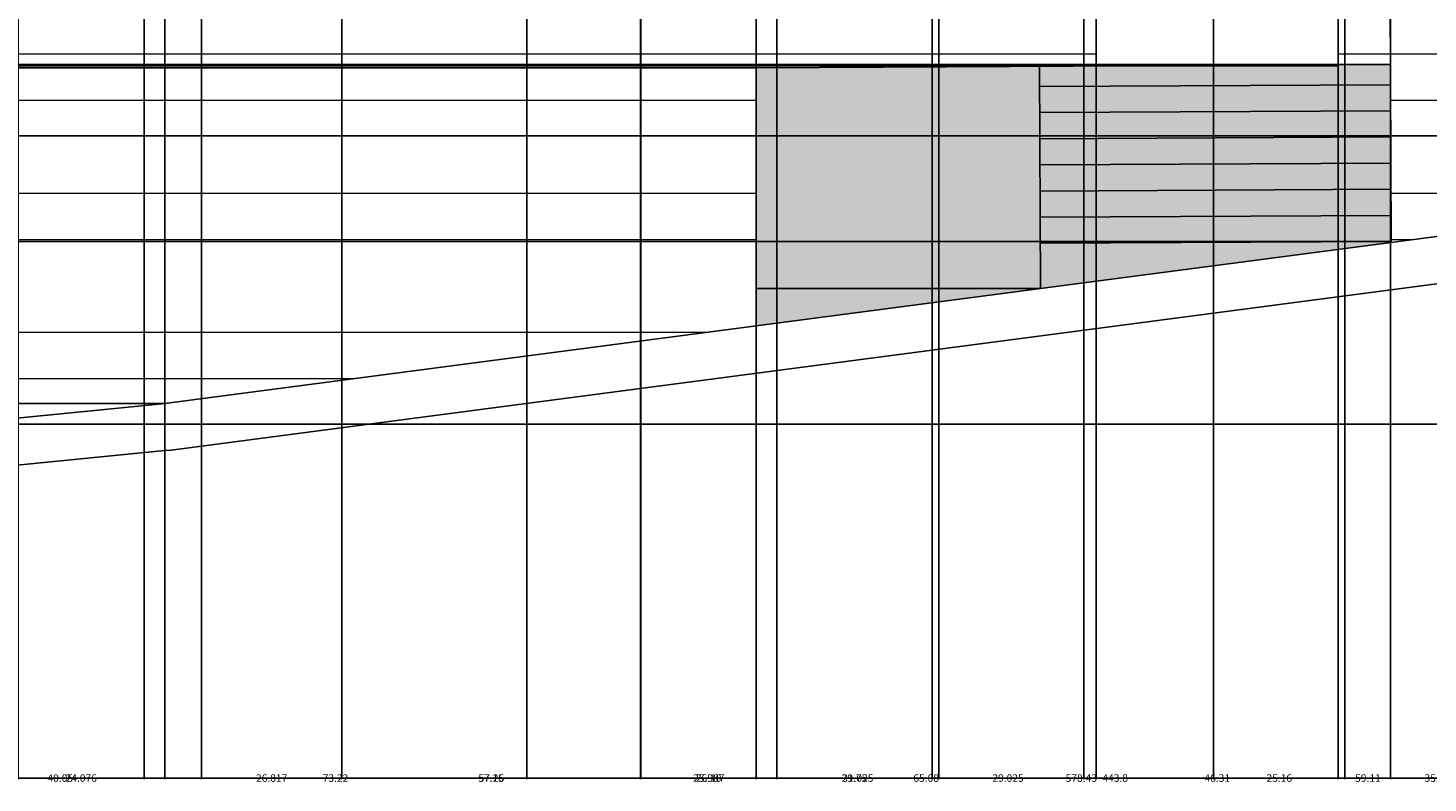
# Model space of a CAD drawing. Units: inches. Extents: x 241 to 943, y 109 to 1396.
# Tile 2 of 34: x 391 to 659, y 109 to 253. Entities that reach past the tile are written whole.
import ezdxf

# ---------------------------------------------------------------- set-up
doc = ezdxf.new("R2010")
doc.units = ezdxf.units.IN
doc.header["$MEASUREMENT"] = 0
for name, color, linetype, lineweight in [('A-ANNO-DIMS', 2, 'Continuous', 18), ('A-ELEV', 7, 'Continuous', 25), ('A-ELEV-SHAD', 9, 'Continuous', 13), ('A-GLAZ', 4, 'Continuous', 18), ('A-WALL-PATT', 8, 'Continuous', 13)]:
    doc.layers.add(name, color=color, linetype=linetype, lineweight=lineweight)
doc.styles.get("Standard").update_dxf_attribs({"font": 'arial.ttf'})
doc.dimstyles.get("Standard").update_dxf_attribs({"dimtxt": 1.4375, "dimasz": 0.18, "dimexe": 0.18, "dimexo": 0.0625, "dimgap": 0.09, "dimtad": 0, "dimtih": 1, "dimtoh": 1, "dimdec": 4, "dimzin": 0, "dimdsep": 46, "dimlunit": 4, "dimtxsty": 'Standard', "dimcen": 0.09, "dimadec": 0, "dimazin": 0, "dimtfac": 1, "dimtdec": 4, "dimtofl": 0, "dimtmove": 0, "dimatfit": 3, "dimfxl": 1, "dimtolj": 1, "dimtzin": 0, "dimarcsym": 0})

# ---------------------------------------------------------------- blocks, each defined once
blk = doc.blocks.new('*D4')
at = {"layer": 'A-ANNO-DIMS', "color": 0, "lineweight": -2, "transparency": 16777216}
for p, q in [((820.84, 232.77), (820.84, 109.81)), ((377.04, 177.64), (377.04, 109.81)), ((377.22, 109.99), (596.39, 109.99)), ((820.66, 109.99), (601.48, 109.99))]:
    blk.add_line(p, q, dxfattribs=at)
at = {"layer": 'A-ANNO-DIMS', "color": 0, "transparency": 16777216}
for points in [[(377.22, 110.02), (377.22, 109.96), (377.04, 109.99)], [(820.66, 110.02), (820.66, 109.96), (820.84, 109.99)]]:
    blk.add_solid(points, dxfattribs=at)
at = {"layer": 'Defpoints', "color": 0, "transparency": 16777216}
for p in [(820.84, 232.83), (377.04, 177.7), (820.84, 109.99)]:
    blk.add_point(p, dxfattribs=at)
at = {"layer": 'A-ANNO-DIMS', "color": 0, "transparency": 16777216, "insert": (598.94, 109.99), "char_height": 1.438, "attachment_point": 5}
blk.add_mtext('\\A1;443.8', dxfattribs=at)
blk = doc.blocks.new('*D7')
at = {"layer": 'A-ANNO-DIMS', "color": 0, "lineweight": -2, "transparency": 16777216}
for p, q in [((508.24, 1336.12), (244.31, 1336.12)), ((244.49, 1335.94), (244.49, 753.25)), ((244.49, 168.92), (244.49, 751.6)), ((303.17, 168.74), (244.31, 168.74))]:
    blk.add_line(p, q, dxfattribs=at)
at = {"layer": 'A-ANNO-DIMS', "color": 0, "transparency": 16777216}
for points in [[(244.46, 1335.94), (244.52, 1335.94), (244.49, 1336.12)], [(244.46, 168.92), (244.52, 168.92), (244.49, 168.74)]]:
    blk.add_solid(points, dxfattribs=at)
at = {"layer": 'Defpoints', "color": 0, "transparency": 16777216}
for p in [(244.49, 1336.12), (508.31, 1336.12), (303.24, 168.74)]:
    blk.add_point(p, dxfattribs=at)
at = {"layer": 'A-ANNO-DIMS', "color": 0, "transparency": 16777216, "insert": (244.49, 752.43), "char_height": 1.438, "attachment_point": 5}
blk.add_mtext('\\A1;1167.4', dxfattribs=at)
blk = doc.blocks.new('*D16')
at = {"layer": 'A-ANNO-DIMS', "color": 0, "lineweight": -2, "transparency": 16777216}
for p, q in [((595.31, 372.88), (595.31, 109.81)), ((641.62, 372.88), (641.62, 109.81)), ((595.49, 109.99), (616.06, 109.99)), ((641.44, 109.99), (620.87, 109.99))]:
    blk.add_line(p, q, dxfattribs=at)
at = {"layer": 'A-ANNO-DIMS', "color": 0, "transparency": 16777216}
for points in [[(595.49, 110.02), (595.49, 109.96), (595.31, 109.99)], [(641.44, 110.02), (641.44, 109.96), (641.62, 109.99)]]:
    blk.add_solid(points, dxfattribs=at)
at = {"layer": 'Defpoints', "color": 0, "transparency": 16777216}
for p in [(595.31, 372.94), (641.62, 372.94), (641.62, 109.99)]:
    blk.add_point(p, dxfattribs=at)
at = {"layer": 'A-ANNO-DIMS', "color": 0, "transparency": 16777216, "insert": (618.47, 109.99), "char_height": 1.438, "attachment_point": 5}
blk.add_mtext('\\A1;46.31', dxfattribs=at)
blk = doc.blocks.new('*D41')
at = {"layer": 'A-ANNO-DIMS', "color": 0, "lineweight": -2, "transparency": 16777216}
for p, q in [((820.77, 400.83), (244.31, 400.83)), ((244.49, 400.65), (244.49, 317.65)), ((244.49, 233.01), (244.49, 316.01)), ((820.77, 232.83), (244.31, 232.83))]:
    blk.add_line(p, q, dxfattribs=at)
at = {"layer": 'A-ANNO-DIMS', "color": 0, "transparency": 16777216}
for points in [[(244.46, 400.65), (244.52, 400.65), (244.49, 400.83)], [(244.46, 233.01), (244.52, 233.01), (244.49, 232.83)]]:
    blk.add_solid(points, dxfattribs=at)
at = {"layer": 'Defpoints', "color": 0, "transparency": 16777216}
for p in [(244.49, 400.83), (820.84, 400.83), (820.84, 232.83)]:
    blk.add_point(p, dxfattribs=at)
at = {"layer": 'A-ANNO-DIMS', "color": 0, "transparency": 16777216, "insert": (244.49, 316.83), "char_height": 1.438, "attachment_point": 5}
blk.add_mtext('\\A1;168', dxfattribs=at)
blk = doc.blocks.new('*D50')
at = {"layer": 'A-ANNO-DIMS', "color": 0, "lineweight": -2, "transparency": 16777216}
for p, q in [((651.55, 246.46), (244.31, 246.46)), ((244.49, 246.28), (244.49, 230.36)), ((244.49, 212.79), (244.49, 228.71)), ((651.72, 212.61), (244.31, 212.61))]:
    blk.add_line(p, q, dxfattribs=at)
at = {"layer": 'A-ANNO-DIMS', "color": 0, "transparency": 16777216}
for points in [[(244.46, 246.28), (244.52, 246.28), (244.49, 246.46)], [(244.46, 212.79), (244.52, 212.79), (244.49, 212.61)]]:
    blk.add_solid(points, dxfattribs=at)
at = {"layer": 'Defpoints', "color": 0, "transparency": 16777216}
for p in [(244.49, 246.46), (651.61, 246.46), (651.79, 212.61)]:
    blk.add_point(p, dxfattribs=at)
at = {"layer": 'A-ANNO-DIMS', "color": 0, "transparency": 16777216, "insert": (244.49, 229.54), "char_height": 1.438, "attachment_point": 5}
blk.add_mtext('\\A1;33.844', dxfattribs=at)
blk = doc.blocks.new('*D51')
at = {"layer": 'A-ANNO-DIMS', "color": 0, "lineweight": -2, "transparency": 16777216}
for p, q in [((595.25, 372.94), (244.31, 372.94)), ((244.49, 372.76), (244.49, 310.39)), ((244.49, 246.38), (244.49, 308.74)), ((595.25, 246.2), (244.31, 246.2))]:
    blk.add_line(p, q, dxfattribs=at)
at = {"layer": 'A-ANNO-DIMS', "color": 0, "transparency": 16777216}
for points in [[(244.46, 372.76), (244.52, 372.76), (244.49, 372.94)], [(244.46, 246.38), (244.52, 246.38), (244.49, 246.2)]]:
    blk.add_solid(points, dxfattribs=at)
at = {"layer": 'Defpoints', "color": 0, "transparency": 16777216}
for p in [(244.49, 372.94), (595.31, 372.94), (595.31, 246.2)]:
    blk.add_point(p, dxfattribs=at)
at = {"layer": 'A-ANNO-DIMS', "color": 0, "transparency": 16777216, "insert": (244.49, 309.57), "char_height": 1.438, "attachment_point": 5}
blk.add_mtext('\\A1;126.74', dxfattribs=at)
blk = doc.blocks.new('*D52')
at = {"layer": 'A-ANNO-DIMS', "color": 0, "lineweight": -2, "transparency": 16777216}
for p, q in [((530.17, 384.18), (244.31, 384.18)), ((244.49, 384), (244.49, 315.83)), ((244.49, 246.02), (244.49, 314.18)), ((530.17, 245.84), (244.31, 245.84))]:
    blk.add_line(p, q, dxfattribs=at)
at = {"layer": 'A-ANNO-DIMS', "color": 0, "transparency": 16777216}
for points in [[(244.46, 384), (244.52, 384), (244.49, 384.18)], [(244.46, 246.02), (244.52, 246.02), (244.49, 245.84)]]:
    blk.add_solid(points, dxfattribs=at)
at = {"layer": 'Defpoints', "color": 0, "transparency": 16777216}
for p in [(244.49, 384.18), (530.23, 384.18), (530.23, 245.84)]:
    blk.add_point(p, dxfattribs=at)
at = {"layer": 'A-ANNO-DIMS', "color": 0, "transparency": 16777216, "insert": (244.49, 315.01), "char_height": 1.438, "attachment_point": 5}
blk.add_mtext('\\A1;138.34', dxfattribs=at)
blk = doc.blocks.new('*D74')
at = {"layer": 'A-ANNO-DIMS', "color": 0, "lineweight": -2, "transparency": 16777216}
for p, q in [((417.09, 181.59), (417.09, 109.81)), ((377.04, 177.64), (377.04, 109.81)), ((377.22, 109.99), (394.52, 109.99)), ((416.91, 109.99), (399.61, 109.99))]:
    blk.add_line(p, q, dxfattribs=at)
at = {"layer": 'A-ANNO-DIMS', "color": 0, "transparency": 16777216}
for points in [[(377.22, 110.02), (377.22, 109.96), (377.04, 109.99)], [(416.91, 110.02), (416.91, 109.96), (417.09, 109.99)]]:
    blk.add_solid(points, dxfattribs=at)
at = {"layer": 'Defpoints', "color": 0, "transparency": 16777216}
for p in [(417.09, 181.65), (377.04, 177.7), (417.09, 109.99)]:
    blk.add_point(p, dxfattribs=at)
at = {"layer": 'A-ANNO-DIMS', "color": 0, "transparency": 16777216, "insert": (397.07, 109.99), "char_height": 1.438, "attachment_point": 5}
blk.add_mtext('\\A1;40.05', dxfattribs=at)
blk = doc.blocks.new('*D75')
at = {"layer": 'A-ANNO-DIMS', "color": 0, "lineweight": -2, "transparency": 16777216}
for p, q in [((667.46, 214.52), (940.6, 214.52)), ((940.42, 214.34), (940.42, 196.93)), ((940.42, 177.88), (940.42, 195.28)), ((377.1, 177.7), (940.6, 177.7))]:
    blk.add_line(p, q, dxfattribs=at)
at = {"layer": 'A-ANNO-DIMS', "color": 0, "transparency": 16777216}
for points in [[(940.39, 214.34), (940.45, 214.34), (940.42, 214.52)], [(940.39, 177.88), (940.45, 177.88), (940.42, 177.7)]]:
    blk.add_solid(points, dxfattribs=at)
at = {"layer": 'Defpoints', "color": 0, "transparency": 16777216}
for p in [(667.39, 214.52), (940.42, 214.52), (377.04, 177.7)]:
    blk.add_point(p, dxfattribs=at)
at = {"layer": 'A-ANNO-DIMS', "color": 0, "transparency": 16777216, "insert": (940.42, 196.11), "char_height": 1.438, "attachment_point": 5}
blk.add_mtext('\\A1;36.82', dxfattribs=at)
blk = doc.blocks.new('*D80')
at = {"layer": 'A-ANNO-DIMS', "color": 0, "lineweight": -2, "transparency": 16777216}
for p, q in [((530.23, 384.12), (530.23, 109.81)), ((595.31, 372.88), (595.31, 109.81)), ((530.41, 109.99), (560.25, 109.99)), ((595.13, 109.99), (565.29, 109.99))]:
    blk.add_line(p, q, dxfattribs=at)
at = {"layer": 'A-ANNO-DIMS', "color": 0, "transparency": 16777216}
for points in [[(530.41, 110.02), (530.41, 109.96), (530.23, 109.99)], [(595.13, 110.02), (595.13, 109.96), (595.31, 109.99)]]:
    blk.add_solid(points, dxfattribs=at)
at = {"layer": 'Defpoints', "color": 0, "transparency": 16777216}
for p in [(530.23, 384.18), (595.31, 372.94), (595.31, 109.99)]:
    blk.add_point(p, dxfattribs=at)
at = {"layer": 'A-ANNO-DIMS', "color": 0, "transparency": 16777216, "insert": (562.77, 109.99), "char_height": 1.438, "attachment_point": 5}
blk.add_mtext('\\A1;65.08', dxfattribs=at)
blk = doc.blocks.new('*D81')
at = {"layer": 'A-ANNO-DIMS', "color": 0, "lineweight": -2, "transparency": 16777216}
for p, q in [((462.04, 274.35), (244.31, 274.35)), ((244.49, 274.17), (244.49, 260.92)), ((244.49, 246.02), (244.49, 259.27)), ((530.17, 245.84), (244.31, 245.84))]:
    blk.add_line(p, q, dxfattribs=at)
at = {"layer": 'A-ANNO-DIMS', "color": 0, "transparency": 16777216}
for points in [[(244.46, 274.17), (244.52, 274.17), (244.49, 274.35)], [(244.46, 246.02), (244.52, 246.02), (244.49, 245.84)]]:
    blk.add_solid(points, dxfattribs=at)
at = {"layer": 'Defpoints', "color": 0, "transparency": 16777216}
for p in [(244.49, 274.35), (462.11, 274.35), (530.23, 245.84)]:
    blk.add_point(p, dxfattribs=at)
at = {"layer": 'A-ANNO-DIMS', "color": 0, "transparency": 16777216, "insert": (244.49, 260.09), "char_height": 1.438, "attachment_point": 5}
blk.add_mtext('\\A1;28.51', dxfattribs=at)
blk = doc.blocks.new('*D97')
at = {"layer": 'A-ANNO-DIMS', "color": 0, "lineweight": -2, "transparency": 16777216}
for p, q in [((881.67, 223.77), (881.67, 109.81)), ((303.24, 168.68), (303.24, 109.81)), ((303.42, 109.99), (589.38, 109.99)), ((881.49, 109.99), (595.53, 109.99))]:
    blk.add_line(p, q, dxfattribs=at)
at = {"layer": 'A-ANNO-DIMS', "color": 0, "transparency": 16777216}
for points in [[(303.42, 110.02), (303.42, 109.96), (303.24, 109.99)], [(881.49, 110.02), (881.49, 109.96), (881.67, 109.99)]]:
    blk.add_solid(points, dxfattribs=at)
at = {"layer": 'Defpoints', "color": 0, "transparency": 16777216}
for p in [(881.67, 223.83), (303.24, 168.74), (881.67, 109.99)]:
    blk.add_point(p, dxfattribs=at)
at = {"layer": 'A-ANNO-DIMS', "color": 0, "transparency": 16777216, "insert": (592.45, 109.99), "char_height": 1.438, "attachment_point": 5}
blk.add_mtext('\\A1;578.43', dxfattribs=at)
blk = doc.blocks.new('*D98')
at = {"layer": 'A-ANNO-DIMS', "color": 0, "lineweight": -2, "transparency": 16777216}
for p, q in [((417.03, 181.65), (244.31, 181.65)), ((244.49, 181.47), (244.49, 180.5)), ((376.98, 177.7), (244.31, 177.7)), ((244.49, 177.88), (244.49, 178.85))]:
    blk.add_line(p, q, dxfattribs=at)
at = {"layer": 'A-ANNO-DIMS', "color": 0, "transparency": 16777216}
for points in [[(244.46, 181.47), (244.52, 181.47), (244.49, 181.65)], [(244.46, 177.88), (244.52, 177.88), (244.49, 177.7)]]:
    blk.add_solid(points, dxfattribs=at)
at = {"layer": 'Defpoints', "color": 0, "transparency": 16777216}
for p in [(244.49, 181.65), (417.09, 181.65), (377.04, 177.7)]:
    blk.add_point(p, dxfattribs=at)
at = {"layer": 'A-ANNO-DIMS', "color": 0, "transparency": 16777216, "insert": (244.49, 179.67), "char_height": 1.438, "attachment_point": 5}
blk.add_mtext('\\A1;3.951', dxfattribs=at)
blk = doc.blocks.new('*D99')
at = {"layer": 'A-ANNO-DIMS', "color": 0, "lineweight": -2, "transparency": 16777216}
for p, q in [((417.09, 181.71), (417.09, 1395.05)), ((417.27, 1394.87), (539.16, 1394.87)), ((667.21, 1394.87), (545.33, 1394.87)), ((667.39, 214.58), (667.39, 1395.05))]:
    blk.add_line(p, q, dxfattribs=at)
at = {"layer": 'A-ANNO-DIMS', "color": 0, "transparency": 16777216}
for points in [[(417.27, 1394.9), (417.27, 1394.84), (417.09, 1394.87)], [(667.21, 1394.9), (667.21, 1394.84), (667.39, 1394.87)]]:
    blk.add_solid(points, dxfattribs=at)
at = {"layer": 'Defpoints', "color": 0, "transparency": 16777216}
for p in [(667.39, 1394.87), (667.39, 214.52), (417.09, 181.65)]:
    blk.add_point(p, dxfattribs=at)
at = {"layer": 'A-ANNO-DIMS', "color": 0, "transparency": 16777216, "insert": (542.24, 1394.87), "char_height": 1.438, "attachment_point": 5}
blk.add_mtext('\\A1;250.30', dxfattribs=at)
blk = doc.blocks.new('*D119')
at = {"layer": 'A-ANNO-DIMS', "color": 0, "lineweight": -2, "transparency": 16777216}
for p, q in [((617.76, 734.79), (617.76, 109.81)), ((642.92, 734.79), (642.92, 109.81)), ((617.94, 109.99), (627.81, 109.99)), ((642.74, 109.99), (632.87, 109.99))]:
    blk.add_line(p, q, dxfattribs=at)
at = {"layer": 'A-ANNO-DIMS', "color": 0, "transparency": 16777216}
for points in [[(617.94, 110.02), (617.94, 109.96), (617.76, 109.99)], [(642.74, 110.02), (642.74, 109.96), (642.92, 109.99)]]:
    blk.add_solid(points, dxfattribs=at)
at = {"layer": 'Defpoints', "color": 0, "transparency": 16777216}
for p in [(617.76, 734.85), (642.92, 734.85), (642.92, 109.99)]:
    blk.add_point(p, dxfattribs=at)
at = {"layer": 'A-ANNO-DIMS', "color": 0, "transparency": 16777216, "insert": (630.34, 109.99), "char_height": 1.438, "attachment_point": 5}
blk.add_mtext('\\A1;25.16', dxfattribs=at)
blk = doc.blocks.new('*D120')
at = {"layer": 'A-ANNO-DIMS', "color": 0, "lineweight": -2, "transparency": 16777216}
for p, q in [((642.92, 734.79), (642.92, 109.81)), ((678.27, 734.79), (678.27, 109.81)), ((643.1, 109.99), (658.07, 109.99)), ((678.09, 109.99), (663.11, 109.99))]:
    blk.add_line(p, q, dxfattribs=at)
at = {"layer": 'A-ANNO-DIMS', "color": 0, "transparency": 16777216}
for points in [[(643.1, 110.02), (643.1, 109.96), (642.92, 109.99)], [(678.09, 110.02), (678.09, 109.96), (678.27, 109.99)]]:
    blk.add_solid(points, dxfattribs=at)
at = {"layer": 'Defpoints', "color": 0, "transparency": 16777216}
for p in [(642.92, 734.85), (678.27, 734.85), (678.27, 109.99)]:
    blk.add_point(p, dxfattribs=at)
at = {"layer": 'A-ANNO-DIMS', "color": 0, "transparency": 16777216, "insert": (660.59, 109.99), "char_height": 1.438, "attachment_point": 5}
blk.add_mtext('\\A1;35.35', dxfattribs=at)
blk = doc.blocks.new('*D126')
at = {"layer": 'A-ANNO-DIMS', "color": 0, "lineweight": -2, "transparency": 16777216}
for p, q in [((450.93, 651.27), (450.93, 109.81)), ((424.11, 628.34), (424.11, 109.81)), ((424.29, 109.99), (434.43, 109.99)), ((450.75, 109.99), (440.6, 109.99))]:
    blk.add_line(p, q, dxfattribs=at)
at = {"layer": 'A-ANNO-DIMS', "color": 0, "transparency": 16777216}
for points in [[(424.29, 110.02), (424.29, 109.96), (424.11, 109.99)], [(450.75, 110.02), (450.75, 109.96), (450.93, 109.99)]]:
    blk.add_solid(points, dxfattribs=at)
at = {"layer": 'Defpoints', "color": 0, "transparency": 16777216}
for p in [(450.93, 651.34), (424.11, 628.4), (450.93, 109.99)]:
    blk.add_point(p, dxfattribs=at)
at = {"layer": 'A-ANNO-DIMS', "color": 0, "transparency": 16777216, "insert": (437.52, 109.99), "char_height": 1.438, "attachment_point": 5}
blk.add_mtext('\\A1;26.817', dxfattribs=at)
blk = doc.blocks.new('*D127')
at = {"layer": 'A-ANNO-DIMS', "color": 0, "lineweight": -2, "transparency": 16777216}
for p, q in [((450.93, 651.27), (450.93, 109.81)), ((508.19, 630.34), (508.19, 109.81)), ((451.11, 109.99), (477.04, 109.99)), ((508.01, 109.99), (482.07, 109.99))]:
    blk.add_line(p, q, dxfattribs=at)
at = {"layer": 'A-ANNO-DIMS', "color": 0, "transparency": 16777216}
for points in [[(451.11, 110.02), (451.11, 109.96), (450.93, 109.99)], [(508.01, 110.02), (508.01, 109.96), (508.19, 109.99)]]:
    blk.add_solid(points, dxfattribs=at)
at = {"layer": 'Defpoints', "color": 0, "transparency": 16777216}
for p in [(450.93, 651.34), (508.19, 630.4), (508.19, 109.99)]:
    blk.add_point(p, dxfattribs=at)
at = {"layer": 'A-ANNO-DIMS', "color": 0, "transparency": 16777216, "insert": (479.56, 109.99), "char_height": 1.438, "attachment_point": 5}
blk.add_mtext('\\A1;57.26', dxfattribs=at)
blk = doc.blocks.new('*D128')
at = {"layer": 'A-ANNO-DIMS', "color": 0, "lineweight": -2, "transparency": 16777216}
for p, q in [((534.18, 651.27), (534.18, 109.81)), ((508.19, 630.34), (508.19, 109.81)), ((508.37, 109.99), (518.1, 109.99)), ((534, 109.99), (524.27, 109.99))]:
    blk.add_line(p, q, dxfattribs=at)
at = {"layer": 'A-ANNO-DIMS', "color": 0, "transparency": 16777216}
for points in [[(508.37, 110.02), (508.37, 109.96), (508.19, 109.99)], [(534, 110.02), (534, 109.96), (534.18, 109.99)]]:
    blk.add_solid(points, dxfattribs=at)
at = {"layer": 'Defpoints', "color": 0, "transparency": 16777216}
for p in [(534.18, 651.34), (508.19, 630.4), (534.18, 109.99)]:
    blk.add_point(p, dxfattribs=at)
at = {"layer": 'A-ANNO-DIMS', "color": 0, "transparency": 16777216, "insert": (521.18, 109.99), "char_height": 1.438, "attachment_point": 5}
blk.add_mtext('\\A1;25.987', dxfattribs=at)
blk = doc.blocks.new('*D129')
at = {"layer": 'A-ANNO-DIMS', "color": 0, "lineweight": -2, "transparency": 16777216}
for p, q in [((534.18, 651.27), (534.18, 109.81)), ((563.93, 651.27), (563.93, 109.81)), ((534.36, 109.99), (546.52, 109.99)), ((563.75, 109.99), (551.59, 109.99))]:
    blk.add_line(p, q, dxfattribs=at)
at = {"layer": 'A-ANNO-DIMS', "color": 0, "transparency": 16777216}
for points in [[(534.36, 110.02), (534.36, 109.96), (534.18, 109.99)], [(563.75, 110.02), (563.75, 109.96), (563.93, 109.99)]]:
    blk.add_solid(points, dxfattribs=at)
at = {"layer": 'Defpoints', "color": 0, "transparency": 16777216}
for p in [(534.18, 651.34), (563.93, 651.34), (563.93, 109.99)]:
    blk.add_point(p, dxfattribs=at)
at = {"layer": 'A-ANNO-DIMS', "color": 0, "transparency": 16777216, "insert": (549.05, 109.99), "char_height": 1.438, "attachment_point": 5}
blk.add_mtext('\\A1;29.75', dxfattribs=at)
blk = doc.blocks.new('*D130')
at = {"layer": 'A-ANNO-DIMS', "color": 0, "lineweight": -2, "transparency": 16777216}
for p, q in [((563.93, 651.27), (563.93, 109.81)), ((592.95, 628.34), (592.95, 109.81)), ((564.11, 109.99), (575.35, 109.99)), ((592.77, 109.99), (581.53, 109.99))]:
    blk.add_line(p, q, dxfattribs=at)
at = {"layer": 'A-ANNO-DIMS', "color": 0, "transparency": 16777216}
for points in [[(564.11, 110.02), (564.11, 109.96), (563.93, 109.99)], [(592.77, 110.02), (592.77, 109.96), (592.95, 109.99)]]:
    blk.add_solid(points, dxfattribs=at)
at = {"layer": 'Defpoints', "color": 0, "transparency": 16777216}
for p in [(563.93, 651.34), (592.95, 628.4), (592.95, 109.99)]:
    blk.add_point(p, dxfattribs=at)
at = {"layer": 'A-ANNO-DIMS', "color": 0, "transparency": 16777216, "insert": (578.44, 109.99), "char_height": 1.438, "attachment_point": 5}
blk.add_mtext('\\A1;29.025', dxfattribs=at)
blk = doc.blocks.new('*D132')
at = {"layer": 'A-ANNO-DIMS', "color": 0, "lineweight": -2, "transparency": 16777216}
for p, q in [((676.87, 628.34), (676.87, 109.81)), ((617.76, 626.34), (617.76, 109.81)), ((617.94, 109.99), (644.94, 109.99)), ((676.69, 109.99), (649.69, 109.99))]:
    blk.add_line(p, q, dxfattribs=at)
at = {"layer": 'A-ANNO-DIMS', "color": 0, "transparency": 16777216}
for points in [[(617.94, 110.02), (617.94, 109.96), (617.76, 109.99)], [(676.69, 110.02), (676.69, 109.96), (676.87, 109.99)]]:
    blk.add_solid(points, dxfattribs=at)
at = {"layer": 'Defpoints', "color": 0, "transparency": 16777216}
for p in [(676.87, 628.4), (617.76, 626.4), (676.87, 109.99)]:
    blk.add_point(p, dxfattribs=at)
at = {"layer": 'A-ANNO-DIMS', "color": 0, "transparency": 16777216, "insert": (647.31, 109.99), "char_height": 1.438, "attachment_point": 5}
blk.add_mtext('\\A1;59.11', dxfattribs=at)
blk = doc.blocks.new('*D136')
at = {"layer": 'A-ANNO-DIMS', "color": 0, "lineweight": -2, "transparency": 16777216}
for p, q in [((450.93, 519.31), (450.93, 109.81)), ((424.11, 496.38), (424.11, 109.81)), ((424.29, 109.99), (434.43, 109.99)), ((450.75, 109.99), (440.6, 109.99))]:
    blk.add_line(p, q, dxfattribs=at)
at = {"layer": 'A-ANNO-DIMS', "color": 0, "transparency": 16777216}
for points in [[(424.29, 110.02), (424.29, 109.96), (424.11, 109.99)], [(450.75, 110.02), (450.75, 109.96), (450.93, 109.99)]]:
    blk.add_solid(points, dxfattribs=at)
at = {"layer": 'Defpoints', "color": 0, "transparency": 16777216}
for p in [(450.93, 519.38), (424.11, 496.44), (450.93, 109.99)]:
    blk.add_point(p, dxfattribs=at)
at = {"layer": 'A-ANNO-DIMS', "color": 0, "transparency": 16777216, "insert": (437.52, 109.99), "char_height": 1.438, "attachment_point": 5}
blk.add_mtext('\\A1;26.817', dxfattribs=at)
blk = doc.blocks.new('*D137')
at = {"layer": 'A-ANNO-DIMS', "color": 0, "lineweight": -2, "transparency": 16777216}
for p, q in [((450.93, 519.31), (450.93, 109.81)), ((508.08, 508.84), (508.08, 109.81)), ((451.11, 109.99), (476.98, 109.99)), ((507.9, 109.99), (482.02, 109.99))]:
    blk.add_line(p, q, dxfattribs=at)
at = {"layer": 'A-ANNO-DIMS', "color": 0, "transparency": 16777216}
for points in [[(451.11, 110.02), (451.11, 109.96), (450.93, 109.99)], [(507.9, 110.02), (507.9, 109.96), (508.08, 109.99)]]:
    blk.add_solid(points, dxfattribs=at)
at = {"layer": 'Defpoints', "color": 0, "transparency": 16777216}
for p in [(450.93, 519.38), (508.08, 508.91), (508.08, 109.99)]:
    blk.add_point(p, dxfattribs=at)
at = {"layer": 'A-ANNO-DIMS', "color": 0, "transparency": 16777216, "insert": (479.5, 109.99), "char_height": 1.438, "attachment_point": 5}
blk.add_mtext('\\A1;57.15', dxfattribs=at)
blk = doc.blocks.new('*D138')
at = {"layer": 'A-ANNO-DIMS', "color": 0, "lineweight": -2, "transparency": 16777216}
for p, q in [((508.08, 508.84), (508.08, 109.81)), ((534.18, 508.84), (534.18, 109.81)), ((508.26, 109.99), (518.6, 109.99)), ((534, 109.99), (523.65, 109.99))]:
    blk.add_line(p, q, dxfattribs=at)
at = {"layer": 'A-ANNO-DIMS', "color": 0, "transparency": 16777216}
for points in [[(508.26, 110.02), (508.26, 109.96), (508.08, 109.99)], [(534, 110.02), (534, 109.96), (534.18, 109.99)]]:
    blk.add_solid(points, dxfattribs=at)
at = {"layer": 'Defpoints', "color": 0, "transparency": 16777216}
for p in [(508.08, 508.91), (534.18, 508.91), (534.18, 109.99)]:
    blk.add_point(p, dxfattribs=at)
at = {"layer": 'A-ANNO-DIMS', "color": 0, "transparency": 16777216, "insert": (521.13, 109.99), "char_height": 1.438, "attachment_point": 5}
blk.add_mtext('\\A1;26.10', dxfattribs=at)
blk = doc.blocks.new('*D139')
at = {"layer": 'A-ANNO-DIMS', "color": 0, "lineweight": -2, "transparency": 16777216}
for p, q in [((534.18, 508.84), (534.18, 109.81)), ((565.2, 496.38), (565.2, 109.81)), ((534.36, 109.99), (546.61, 109.99)), ((565.02, 109.99), (552.77, 109.99))]:
    blk.add_line(p, q, dxfattribs=at)
at = {"layer": 'A-ANNO-DIMS', "color": 0, "transparency": 16777216}
for points in [[(534.36, 110.02), (534.36, 109.96), (534.18, 109.99)], [(565.02, 110.02), (565.02, 109.96), (565.2, 109.99)]]:
    blk.add_solid(points, dxfattribs=at)
at = {"layer": 'Defpoints', "color": 0, "transparency": 16777216}
for p in [(534.18, 508.91), (565.2, 496.44), (565.2, 109.99)]:
    blk.add_point(p, dxfattribs=at)
at = {"layer": 'A-ANNO-DIMS', "color": 0, "transparency": 16777216, "insert": (549.69, 109.99), "char_height": 1.438, "attachment_point": 5}
blk.add_mtext('\\A1;31.025', dxfattribs=at)
blk = doc.blocks.new('*D142')
at = {"layer": 'A-ANNO-DIMS', "color": 0, "lineweight": -2, "transparency": 16777216}
for p, q in [((689.79, 498.38), (689.79, 109.81)), ((651.6, 496.38), (651.6, 109.81)), ((651.78, 109.99), (668.18, 109.99)), ((689.61, 109.99), (673.21, 109.99))]:
    blk.add_line(p, q, dxfattribs=at)
at = {"layer": 'A-ANNO-DIMS', "color": 0, "transparency": 16777216}
for points in [[(651.78, 110.02), (651.78, 109.96), (651.6, 109.99)], [(689.61, 110.02), (689.61, 109.96), (689.79, 109.99)]]:
    blk.add_solid(points, dxfattribs=at)
at = {"layer": 'Defpoints', "color": 0, "transparency": 16777216}
for p in [(689.79, 498.44), (651.6, 496.44), (689.79, 109.99)]:
    blk.add_point(p, dxfattribs=at)
at = {"layer": 'A-ANNO-DIMS', "color": 0, "transparency": 16777216, "insert": (670.7, 109.99), "char_height": 1.438, "attachment_point": 5}
blk.add_mtext('\\A1;38.20', dxfattribs=at)
blk = doc.blocks.new('*D147')
at = {"layer": 'A-ANNO-DIMS', "color": 0, "lineweight": -2, "transparency": 16777216}
for p, q in [((389.04, 734.79), (389.04, 109.81)), ((413.12, 734.79), (413.12, 109.81)), ((389.22, 109.99), (398, 109.99)), ((412.94, 109.99), (404.17, 109.99))]:
    blk.add_line(p, q, dxfattribs=at)
at = {"layer": 'A-ANNO-DIMS', "color": 0, "transparency": 16777216}
for points in [[(389.22, 110.02), (389.22, 109.96), (389.04, 109.99)], [(412.94, 110.02), (412.94, 109.96), (413.12, 109.99)]]:
    blk.add_solid(points, dxfattribs=at)
at = {"layer": 'Defpoints', "color": 0, "transparency": 16777216}
for p in [(389.04, 734.85), (413.12, 734.85), (413.12, 109.99)]:
    blk.add_point(p, dxfattribs=at)
at = {"layer": 'A-ANNO-DIMS', "color": 0, "transparency": 16777216, "insert": (401.08, 109.99), "char_height": 1.438, "attachment_point": 5}
blk.add_mtext('\\A1;24.076', dxfattribs=at)
blk = doc.blocks.new('*D148')
at = {"layer": 'A-ANNO-DIMS', "color": 0, "lineweight": -2, "transparency": 16777216}
for p, q in [((413.12, 734.79), (413.12, 109.81)), ((486.34, 734.79), (486.34, 109.81)), ((413.3, 109.99), (447.23, 109.99)), ((486.16, 109.99), (452.23, 109.99))]:
    blk.add_line(p, q, dxfattribs=at)
at = {"layer": 'A-ANNO-DIMS', "color": 0, "transparency": 16777216}
for points in [[(413.3, 110.02), (413.3, 109.96), (413.12, 109.99)], [(486.16, 110.02), (486.16, 109.96), (486.34, 109.99)]]:
    blk.add_solid(points, dxfattribs=at)
at = {"layer": 'Defpoints', "color": 0, "transparency": 16777216}
for p in [(413.12, 734.85), (486.34, 734.85), (486.34, 109.99)]:
    blk.add_point(p, dxfattribs=at)
at = {"layer": 'A-ANNO-DIMS', "color": 0, "transparency": 16777216, "insert": (449.73, 109.99), "char_height": 1.438, "attachment_point": 5}
blk.add_mtext('\\A1;73.22', dxfattribs=at)

msp = doc.modelspace()

# ---------------------------------------------------------------- hatches: boundary and pattern name
at = {"layer": 'A-ELEV-SHAD'}
h = msp.add_hatch(color=256, dxfattribs=at)
h.dxf.hatch_style = 1
h.paths.add_polyline_path([(584.4646, 246.1155), (530.2303, 245.8378), (530.2303, 203.6623), (584.682, 203.6572)])
h.paths.add_polyline_path([(584.682, 203.6572), (530.2303, 203.6623), (530.2303, 196.5065)])
h = msp.add_hatch(color=256, dxfattribs=at)
h.dxf.hatch_style = 1
h.paths.add_polyline_path([(651.6121, 246.4593), (641.6196, 246.4081), (641.6196, 246.1966), (600.309, 246.1966), (584.4646, 246.1155), (584.4843, 242.2707), (651.6318, 242.6145)])
h.paths.add_polyline_path([(651.6318, 242.6145), (584.4843, 242.2707), (584.5099, 237.2707), (651.6574, 237.6145)])
h.paths.add_polyline_path([(651.6574, 237.6145), (584.5099, 237.2707), (584.5355, 232.2708), (651.683, 232.6146)])
h.paths.add_polyline_path([(651.683, 232.6146), (584.5355, 232.2708), (584.5611, 227.2709), (651.7086, 227.6147)])
h.paths.add_polyline_path([(651.7086, 227.6147), (584.5611, 227.2709), (584.5867, 222.2709), (651.7342, 222.6147)])
h.paths.add_polyline_path([(651.7342, 222.6147), (584.5867, 222.2709), (584.6123, 217.271), (651.7598, 217.6148)])
h.paths.add_polyline_path([(651.7598, 217.6148), (584.6123, 217.271), (584.6379, 212.2711), (651.7854, 212.6149)])
h.paths.add_polyline_path([(651.7861, 212.4693), (651.7854, 212.6149), (584.6379, 212.2711), (584.682, 203.6572)])
at = {"layer": 'A-WALL-PATT'}
h = msp.add_hatch(dxfattribs=at)
h.set_pattern_fill('ANSI32', color=256, scale=71, angle=135)
h.paths.add_polyline_path([(820.8374, 568.8295), (792.691, 568.8295), (792.691, 496.4395), (651.5974, 496.4395), (651.5974, 568.8295), (617.7594, 568.8295), (618.9643, 400.8295), (417.0913, 400.8295), (377.0391, 400.8295), (377.0391, 398.8538), (377.0391, 396.8782), (377.0391, 228.8782), (377.0391, 177.6977), (416.5078, 181.5724), (417.0913, 181.649), (530.2303, 196.5065), (530.2303, 384.1784), (650.907, 384.1784), (651.7861, 212.4693), (667.3935, 214.5189), (667.3935, 289.9984), (794.0275, 289.9984), (794.0275, 232.8295), (820.8374, 232.8295), (820.8374, 400.8295)])
h.paths.add_polyline_path([(500.3323, 384.1784), (500.3323, 289.6933), (500.3323, 274.3507), (479.596, 274.3507), (479.596, 289.6933), (479.596, 384.1784)], flags=16)
h.paths.add_polyline_path([(498.3323, 382.1784), (498.3323, 291.6933), (481.596, 291.6933), (481.596, 382.1784)], flags=0)
h.paths.add_polyline_path([(462.1074, 384.1784), (462.1074, 289.6933), (462.1074, 277.4626), (462.1074, 274.3507), (390.895, 274.3507), (390.895, 277.4626), (390.895, 289.6933), (390.895, 384.1784)], flags=16)
h.paths.add_polyline_path([(460.1074, 382.1784), (460.1074, 291.6933), (392.895, 291.6933), (392.895, 382.1784)], flags=0)
h.paths.add_polyline_path([(595.3136, 372.9401), (641.6196, 372.9401), (641.6196, 246.4081), (651.6121, 246.4593), (650.907, 384.1784), (530.2303, 384.1784), (530.2303, 245.8378), (595.3136, 246.1711)], flags=17)

# ---------------------------------------------------------------- linework, layer by layer
at = {"layer": 'A-ELEV'}
for p, q in [((530.2303, 196.5065), (530.2303, 384.1784)), ((650.907, 384.1784), (651.7861, 212.4693)), ((530.2303, 245.8378), (651.6121, 246.4593)), ((584.682, 203.6572), (584.4646, 246.1155)), ((584.4843, 242.2707), (651.6318, 242.6145)), ((584.5099, 237.2707), (651.6574, 237.6145)), ((584.5355, 232.2708), (651.683, 232.6146)), ((584.5611, 227.2709), (651.7086, 227.6147)), ((584.5867, 222.2709), (651.7342, 222.6147)), ((584.6123, 217.271), (651.7598, 217.6148)), ((667.3935, 214.5189), (417.0913, 181.649)), ((584.6379, 212.2711), (651.7854, 212.6149)), ((668.5653, 205.5955), (418.2631, 172.7256)), ((530.2303, 203.6623), (584.682, 203.6572)), ((416.5078, 181.5724), (377.0391, 177.6977)), ((416.5078, 181.5724), (417.0913, 181.649)), ((417.0913, 172.649), (377.9184, 168.7407)), ((417.0913, 172.649), (418.2631, 172.7256))]:
    msp.add_line(p, q, dxfattribs=at)
at = {"layer": 'A-GLAZ'}
msp.add_lwpolyline([(595.3136, 246.1966), (641.6196, 246.1966), (641.6196, 372.9401), (595.3136, 372.9401)], close=True, dxfattribs=at)

# ---------------------------------------------------------------- dimensions: what is measured, and where the dimension line sits
at = {"layer": 'A-ANNO-DIMS'}
for base, p1, p2, override, picture, middle in [((667.3935, 1394.8654), (417.0913, 181.649), (667.3935, 214.5189), {"dimdec": 2, "dimlfac": 1, "dimrnd": 0, "dimzin": 0, "dimdsep": 46, "dimlunit": 2}, '*D99', (542.2424, 1394.8654)), ((413.1187, 109.9907), (389.0429, 734.8538), (413.1187, 734.8538), {"dimdec": 3, "dimlfac": 1, "dimrnd": 0, "dimzin": 0, "dimdsep": 46, "dimlunit": 2}, '*D147', (401.0808, 109.9907)), ((486.3418, 109.9907), (413.1187, 734.8538), (486.3418, 734.8538), {"dimdec": 2, "dimlfac": 1, "dimrnd": 0, "dimzin": 0, "dimdsep": 46, "dimlunit": 2}, '*D148', (449.7303, 109.9907)), ((642.9197, 109.9907), (617.7594, 734.8538), (642.9197, 734.8538), {"dimdec": 2, "dimlfac": 1, "dimrnd": 0, "dimzin": 0, "dimdsep": 46, "dimlunit": 2}, '*D119', (630.3395, 109.9907)), ((678.2674, 109.9907), (642.9197, 734.8538), (678.2674, 734.8538), {"dimdec": 2, "dimlfac": 1, "dimrnd": 0, "dimzin": 0, "dimdsep": 46, "dimlunit": 2}, '*D120', (660.5935, 109.9907)), ((450.9259, 109.9907), (424.1086, 628.4013), (450.9259, 651.3371), {"dimdec": 3, "dimlfac": 1, "dimrnd": 0, "dimzin": 0, "dimdsep": 46, "dimlunit": 2}, '*D126', (437.5172, 109.9907)), ((508.1906, 109.9907), (450.9259, 651.3371), (508.1906, 630.4013), {"dimdec": 2, "dimlfac": 1, "dimrnd": 0, "dimzin": 0, "dimdsep": 46, "dimlunit": 2}, '*D127', (479.5582, 109.9907)), ((534.1778, 109.9907), (508.1906, 630.4013), (534.1778, 651.3371), {"dimdec": 3, "dimlfac": 1, "dimrnd": 0, "dimzin": 0, "dimdsep": 46, "dimlunit": 2}, '*D128', (521.1842, 109.9907)), ((563.9297, 109.9907), (534.1778, 651.3371), (563.9297, 651.3371), {"dimdec": 2, "dimlfac": 1, "dimrnd": 0, "dimzin": 0, "dimdsep": 46, "dimlunit": 2}, '*D129', (549.0538, 109.9907)), ((592.954223, 109.990742), (563.92972, 651.337109), (592.954223, 628.401255), {"dimdec": 3, "dimlfac": 1, "dimrnd": 0, "dimzin": 0, "dimdsep": 46, "dimlunit": 2}, '*D130', (578.441971, 109.990742)), ((676.8698, 109.9907), (617.7594, 626.4013), (676.8698, 628.4013), {"dimdec": 2, "dimlfac": 1, "dimrnd": 0, "dimzin": 0, "dimdsep": 46, "dimlunit": 2}, '*D132', (647.3146, 109.9907)), ((450.9259, 109.9907), (424.1086, 496.4395), (450.9259, 519.3754), {"dimdec": 3, "dimlfac": 1, "dimrnd": 0, "dimzin": 0, "dimdsep": 46, "dimlunit": 2}, '*D136', (437.5172, 109.9907)), ((508.0803, 109.9907), (450.9259, 519.3754), (508.0803, 508.9074), {"dimdec": 2, "dimlfac": 1, "dimrnd": 0, "dimzin": 0, "dimdsep": 46, "dimlunit": 2}, '*D137', (479.5031, 109.9907)), ((534.1778, 109.9907), (508.0803, 508.9074), (534.1778, 508.9074), {"dimdec": 2, "dimlfac": 1, "dimrnd": 0, "dimzin": 0, "dimdsep": 46, "dimlunit": 2}, '*D138', (521.1291, 109.9907)), ((565.20229, 109.99074), (534.17778, 508.90744), (565.20229, 496.43952), {"dimdec": 3, "dimlfac": 1, "dimrnd": 0, "dimzin": 0, "dimdsep": 46, "dimlunit": 2}, '*D139', (549.69004, 109.99074)), ((689.794, 109.9907), (651.5974, 496.4395), (689.794, 498.4395), {"dimdec": 2, "dimlfac": 1, "dimrnd": 0, "dimzin": 0, "dimdsep": 46, "dimlunit": 2}, '*D142', (670.6957, 109.9907)), ((595.3136, 109.9907), (530.2303, 384.1784), (595.3136, 372.9401), {"dimdec": 2, "dimlfac": 1, "dimrnd": 0, "dimzin": 0, "dimdsep": 46, "dimlunit": 2}, '*D80', (562.772, 109.9907)), ((641.6196, 109.9907), (595.3136, 372.9401), (641.6196, 372.9401), {"dimdec": 2, "dimlfac": 1, "dimrnd": 0, "dimzin": 0, "dimdsep": 46, "dimlunit": 2}, '*D16', (618.4666, 109.9907)), ((820.8374, 109.9907), (377.0391, 177.6977), (820.8374, 232.8295), {"dimdec": 1, "dimlfac": 1, "dimrnd": 0, "dimzin": 0, "dimdsep": 46, "dimlunit": 2}, '*D4', (598.9383, 109.9907)), ((881.667, 109.9907), (303.2358, 168.7407), (881.667, 223.8295), {"dimdec": 2, "dimlfac": 1, "dimrnd": 0, "dimzin": 0, "dimdsep": 46, "dimlunit": 2}, '*D97', (592.4514, 109.9907)), ((417.0913, 109.9907), (377.0391, 177.6977), (417.0913, 181.649), {"dimdec": 2, "dimlfac": 1, "dimrnd": 0, "dimzin": 0, "dimdsep": 46, "dimlunit": 2}, '*D74', (397.0652, 109.9907))]:
    dim = msp.add_linear_dim(base=base, p1=p1, p2=p2, dimstyle='Standard', override=override, dxfattribs=at)
    dim.commit()
    dim.dimension.update_dxf_attribs({"geometry": picture, "text_midpoint": middle})
for base, p1, p2, override, picture, middle in [((244.4858, 1336.1154), (303.2358, 168.7407), (508.3064, 1336.1154), {"dimdec": 1, "dimlfac": 1, "dimrnd": 0, "dimzin": 0, "dimdsep": 46, "dimlunit": 2}, '*D7', (244.4858, 752.4281)), ((244.4858, 400.8295), (820.8374, 232.8295), (820.8374, 400.8295), {"dimdec": 0, "dimlfac": 1, "dimrnd": 0, "dimzin": 0, "dimdsep": 46, "dimlunit": 2}, '*D41', (244.4858, 316.8295)), ((244.4858, 384.1784), (530.2303, 245.8378), (530.2303, 384.1784), {"dimdec": 2, "dimlfac": 1, "dimrnd": 0, "dimzin": 0, "dimdsep": 46, "dimlunit": 2}, '*D52', (244.4858, 315.0081)), ((244.4858, 372.9401), (595.3136, 246.1966), (595.3136, 372.9401), {"dimdec": 2, "dimlfac": 1, "dimrnd": 0, "dimzin": 0, "dimdsep": 46, "dimlunit": 2}, '*D51', (244.4858, 309.5684)), ((244.4858, 274.3507), (530.2303, 245.8378), (462.1074, 274.3507), {"dimdec": 2, "dimlfac": 1, "dimrnd": 0, "dimzin": 0, "dimdsep": 46, "dimlunit": 2}, '*D81', (244.4858, 260.0943)), ((244.4858, 246.4593), (651.7854, 212.6149), (651.6121, 246.4593), {"dimdec": 3, "dimlfac": 1, "dimrnd": 0, "dimzin": 0, "dimdsep": 46, "dimlunit": 2}, '*D50', (244.4858, 229.5371)), ((940.417, 214.5189), (377.0391, 177.6977), (667.3935, 214.5189), {"dimdec": 2, "dimlfac": 1, "dimrnd": 0, "dimzin": 0, "dimdsep": 46, "dimlunit": 2}, '*D75', (940.417, 196.1083)), ((244.4858, 181.649), (377.0391, 177.6977), (417.0913, 181.649), {"dimdec": 3, "dimlfac": 1, "dimrnd": 0, "dimzin": 0, "dimdsep": 46, "dimlunit": 2}, '*D98', (244.4858, 179.6733))]:
    dim = msp.add_linear_dim(base=base, p1=p1, p2=p2, angle=90, dimstyle='Standard', override=override, dxfattribs=at)
    dim.commit()
    dim.dimension.update_dxf_attribs({"geometry": picture, "text_midpoint": middle})

doc.saveas('drawing.dxf')
